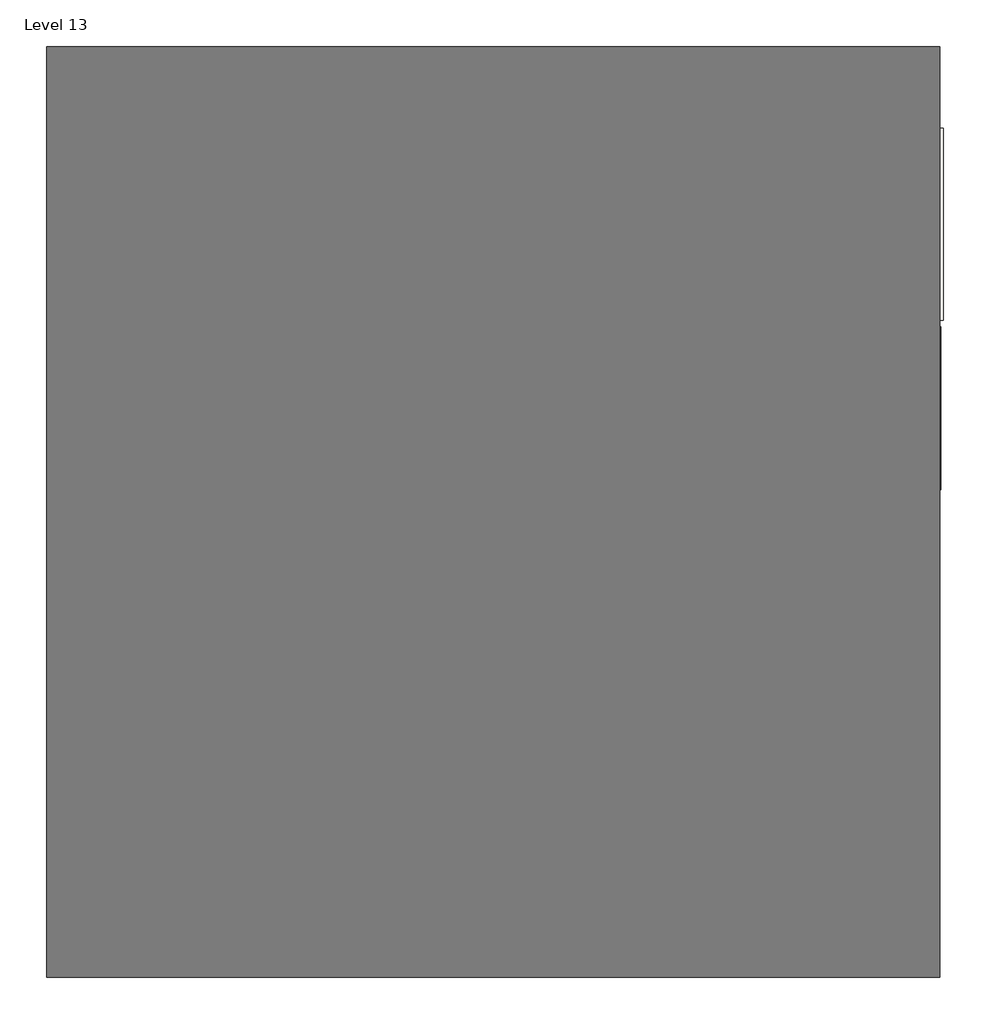
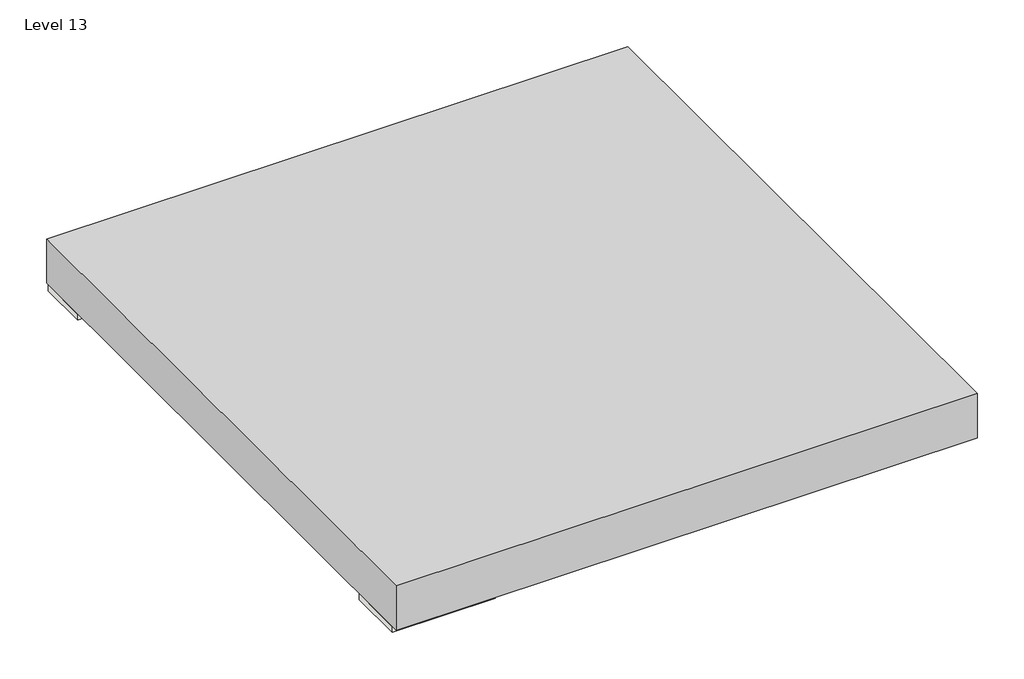
# One storey: 7 slabs, 1 proxy.
"""IFC4 building model written with IfcOpenShell, lengths in millimetres."""

from ifc_helpers import new_model, si_unit, frame, origin, place, context, project, spatial, polyline, outline, extrude, transform, mapped, element, save
from components import generic_models_13_generic_models_13_5b4bef59

model = new_model("IFC4")

# Units and contexts
model_context = context("Model", 3, world=origin())
ifc_project = project(units=[si_unit("LENGTHUNIT", "METRE", prefix="MILLI")], contexts=[model_context])

# Site, building, storey
site = spatial("IfcSite", under=ifc_project)
building = spatial("IfcBuilding", under=site)
storey = spatial("IfcBuildingStorey", under=building, Name="Level 13", Elevation=18897.6)

# Proxy
placement = place(None, origin())
generic_models_13_generic_models_13_shape = generic_models_13_generic_models_13_5b4bef59(model_context)
element("IfcBuildingElementProxy", 1, Name="Generic Models 13 : Generic Models 13", ObjectType="Generic Models 13 : Generic Models 13", at=placement, inside=storey, context=model_context, shape_type="MappedRepresentation", body=[
    mapped(generic_models_13_generic_models_13_shape, transform((0.0, 0.0, 0.0), x_axis=(1.0, 0.0, 0.0), y_axis=(0.0, 1.0, 0.0), z_axis=(0.0, 0.0, 1.0))),
])

# Slabs
element("IfcSlab", 2, ObjectType="Generic - 12\"", at=placement, inside=storey, context=model_context, shape_type="SweptSolid", body=[
    extrude(outline(polyline([(14106.5361222, -10428.1762475), (14106.5361222, -12886.3749501), (2981.3361222, -12886.3749501), (2981.3361222, -10428.1762475), (14106.5361222, -10428.1762475)])), frame((0.0, 0.0, 18592.8), z_axis=(0.0, 0.0, 1.0), x_axis=(1.0, 0.0, 0.0)), (0.0, 0.0, 1.0), 304.8),
])
element("IfcSlab", 3, ObjectType="Generic - 12\"", at=placement, inside=storey, context=model_context, shape_type="SweptSolid", body=[
    extrude(outline(polyline([(2981.3361222, -10428.1762475), (2981.3361222, -12886.3749501), (-4029.0638778, -12886.3749501), (-4029.0638778, -10428.1762475), (2981.3361222, -10428.1762475)])), frame((0.0, 0.0, 18592.8), z_axis=(0.0, 0.0, 1.0), x_axis=(1.0, 0.0, 0.0)), (0.0, 0.0, 1.0), 304.8),
])
element("IfcSlab", 4, ObjectType="Generic - 12\"", at=placement, inside=storey, context=model_context, shape_type="SweptSolid", body=[
    extrude(outline(polyline([(-8499.4638778, -10428.1762475), (-8499.4638778, -13374.5762475), (-13833.4638778, -13374.5762475), (-13833.4638778, -10428.1762475), (-8499.4638778, -10428.1762475)])), frame((0.0, 0.0, 18592.8), z_axis=(0.0, 0.0, 1.0), x_axis=(1.0, 0.0, 0.0)), (0.0, 0.0, 1.0), 304.8),
])
element("IfcSlab", 5, ObjectType="Generic - 12\"", at=placement, inside=storey, context=model_context, shape_type="SweptSolid", body=[
    extrude(outline(polyline([(16240.1361222, 8164.6237525), (16240.1361222, 2678.2237525), (14106.5361222, 2678.2237525), (14106.5361222, 8164.6237525), (16240.1361222, 8164.6237525)])), frame((0.0, 0.0, 18592.8), z_axis=(0.0, 0.0, 1.0), x_axis=(1.0, 0.0, 0.0)), (0.0, 0.0, 1.0), 304.8),
])
element("IfcSlab", 6, ObjectType="Generic - 12\"", at=placement, inside=storey, context=model_context, shape_type="SweptSolid", body=[
    extrude(outline(polyline([(16321.4289933, 14825.1934186), (16321.4289933, 8367.8237525), (14106.5361222, 8367.8237525), (14106.5361222, 14825.1934186), (16321.4289933, 14825.1934186)])), frame((0.0, 0.0, 18592.8), z_axis=(0.0, 0.0, 1.0), x_axis=(1.0, 0.0, 0.0)), (0.0, 0.0, 1.0), 304.8),
])
element("IfcSlab", 7, ObjectType="Generic - 12\"", at=placement, inside=storey, context=model_context, shape_type="SweptSolid", body=[
    extrude(outline(polyline([(13903.3361222, 14768.6237525), (7096.1361222, 14768.6237525), (7096.1361222, 16495.8237525), (13903.3361222, 16495.8237525), (13903.3361222, 14768.6237525)])), frame((0.0, 0.0, 18592.8), z_axis=(0.0, 0.0, 1.0), x_axis=(1.0, 0.0, 0.0)), (0.0, 0.0, 1.0), 304.8),
])
element("IfcSlab", 8, ObjectType="Generic - 12\"", at=placement, inside=storey, context=model_context, shape_type="SweptSolid", body=[
    extrude(outline(polyline([(-13833.4638778, 14768.6237525), (-13833.4638778, 17410.2237525), (-3775.0638778, 17410.2237525), (-3775.0638778, 14768.6237525), (-13833.4638778, 14768.6237525)])), frame((0.0, 0.0, 18592.8), z_axis=(0.0, 0.0, 1.0), x_axis=(1.0, 0.0, 0.0)), (0.0, 0.0, 1.0), 304.8),
])

save(model, "model.ifc")

# Revit data of these elements
# Type "Generic - 12\""
#   Assembly Code = "B1010"
#   Function = 0
#   Layers, outside or top first: 1' - 0" no material (function 1)
# Element 1 (IfcBuildingElementProxy, "Generic Models 13 : Generic Models 13")
#   Phase Created = New Construction
# Elements 2, 3, 4, 5, 6, 7 (IfcSlab, "Generic - 12\"")
#   Height Offset From Level = 0' - 0"
#   Phase Created = New Construction
#   Materials on its faces: "Default Floor"
# Element 8 (IfcSlab, "Generic - 12\"")
#   built-in parameter 1001955 = 3.14159 (stored number, unit not read)
#   Height Offset From Level = 0' - 0"
#   Phase Created = New Construction
#   Materials on its faces: "Default Floor"
# Materials
#   "Default Floor": colour RGB 128 128 128, transparency 0
